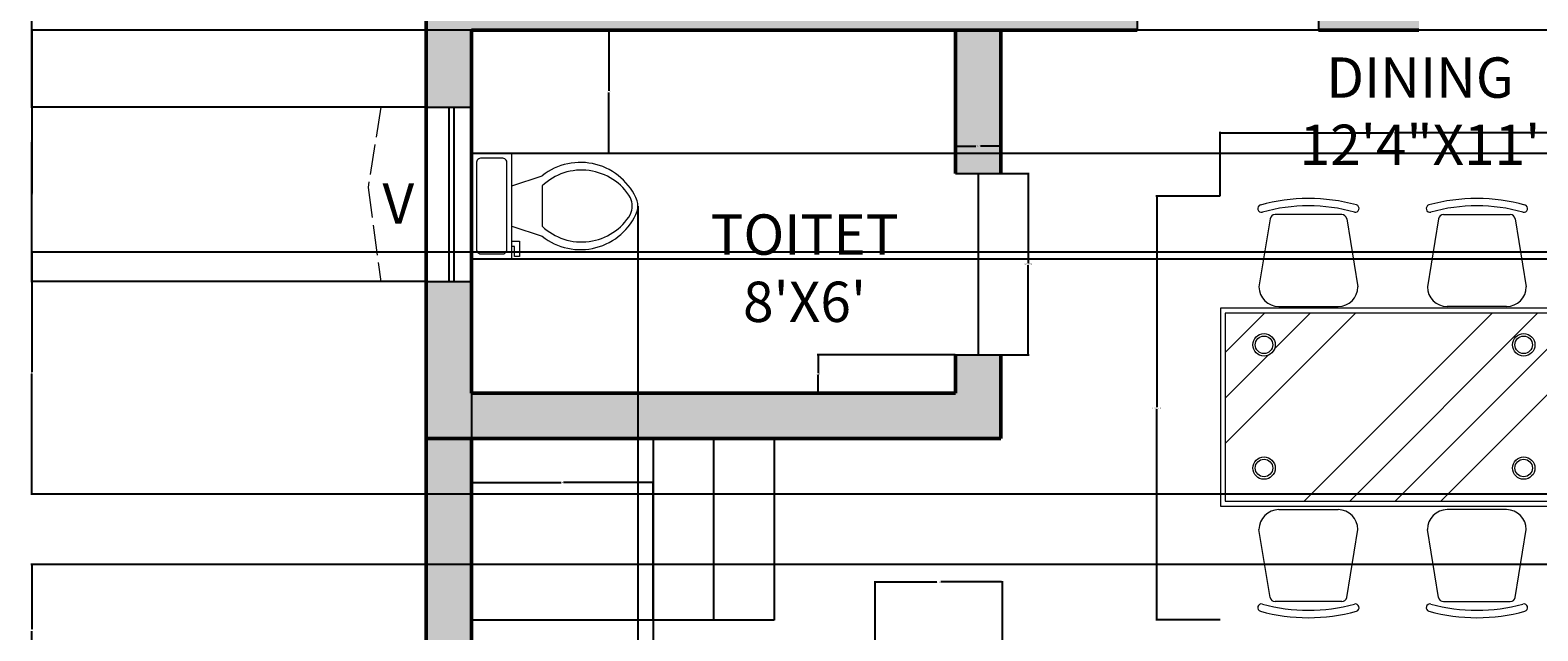
# Model space of a CAD drawing. Units: inches. Extents: x -75 to 416, y -487 to 70.
# Tile 2 of 5: x -75 to 224, y -253 to -133. Entities that reach past the tile are written whole.
import ezdxf

# ---------------------------------------------------------------- set-up
doc = ezdxf.new("R2010")
doc.units = ezdxf.units.IN
doc.header["$MEASUREMENT"] = 0
doc.linetypes.add('ACAD_ISO02W100', pattern=[15, 12, -3])
for name, color, linetype, lineweight in [('A-ANNO-DIMS', 2, 'Continuous', 18), ('A-ANNO-TEXT', 7, 'Continuous', 18), ('A-AREA-IDEN', 7, 'Continuous', 25), ('A-DOOR', 3, 'Continuous', 25), ('A-FLOR-FIXT', 9, 'Continuous', 18), ('A-FLOR-STRS', 7, 'Continuous', 25), ('A-FURN', 8, 'Continuous', 18), ('A-GLAZ', 4, 'Continuous', 25), ('A-GLAZ-OVHD', 4, 'ACAD_ISO02W100', 13), ('A-WALL', 7, 'Continuous', 50), ('A-WALL-PATT', 252, 'Continuous', 13)]:
    doc.layers.add(name, color=color, linetype=linetype, lineweight=lineweight)
doc.styles.get("Standard").update_dxf_attribs({"font": 'arial.ttf'})
doc.dimstyles.get("Standard").update_dxf_attribs({"dimtxt": 0.18, "dimasz": 0.18, "dimexe": 0.18, "dimexo": 0.0625, "dimgap": 0.09, "dimtad": 0, "dimtih": 1, "dimtoh": 1, "dimdec": 4, "dimzin": 0, "dimdsep": 46, "dimtxsty": 'Standard', "dimcen": 0.09, "dimadec": 0, "dimazin": 0, "dimtfac": 1, "dimtdec": 4, "dimtofl": 0, "dimtmove": 0, "dimatfit": 3, "dimfxl": 1, "dimtolj": 1, "dimtzin": 0, "dimarcsym": 0})

# ---------------------------------------------------------------- blocks, each defined once
blk = doc.blocks.new('*U4')
for p, q in [((9.5, -6), (9.5, -2)), ((-10, -8.5), (-8, -8.5)), ((-10, -9.5), (-10, -8.5)), ((-8, -8.5), (-8, -8)), ((-7, -8), (-7, -9.5)), ((-4, -8), (-6, -14)), ((4, -8), (6, -14)), ((-7, -9.5), (-10, -9.5)), ((4, -14), (-4, -14))]:
    blk.add_line(p, q)
blk.add_lwpolyline([(10.5, -8), (10.5, 0), (-10.5, 0), (-10.5, -8)], close=True)
for points in [[(-9.5, -2), (-9.5, -6)], [(8.5, -1), (-8.5, -1)], [(-8.5, -7), (8.5, -7)]]:
    blk.add_lwpolyline(points)
for centre, radius, start, end in [((-8.62, -1.88), 0.884, 81.8699, 188.1301), ((8.62, -1.88), 0.884, 351.8699, 98.1301), ((-8.62, -6.12), 0.884, 171.8699, 278.1301), ((8.62, -6.12), 0.884, 261.8699, 8.1301), ((3.52, -21.58), 12.17, 141.4691, 247.9714), ((4.2, -21.82), 11.33, 136.3677, 238.9468), ((-3.52, -21.58), 12.17, 292.0284, 38.5307), ((-4.2, -21.82), 11.33, 301.053, 43.6321), ((0, -27.88), 4, 245.7318, 294.2682), ((0, -29), 4, 254.8605, 285.1395)]:
    blk.add_arc(centre, radius, start, end)
blk = doc.blocks.new('A$C0FD55737')
for p, q in [((0.2013, 1.6134), (0.1562, 1.3384)), ((0.4912, 1.6302), (0.2211, 1.6302)), ((0.511, 1.6134), (0.5562, 1.3384)), ((0.8828, 1.6134), (0.8376, 1.3384)), ((0.9026, 1.6302), (1.1727, 1.6302)), ((1.1925, 1.6134), (1.2376, 1.3384)), ((0, 1.2513), (0, 0.4513)), ((1.4, 1.2513), (0, 1.2513)), ((0.02, 1.0725), (0.1788, 1.2313)), ((0.02, 0.7043), (0.547, 1.2313)), ((1.38, 1.2313), (0.02, 1.2313)), ((0.02, 1.2313), (0.02, 0.4713)), ((0.2189, 1.0873), (0.3629, 1.2313)), ((0.2362, 1.2584), (0.4762, 1.2584)), ((0.3393, 0.4713), (1.0993, 1.2313)), ((0.5234, 0.4713), (1.2834, 1.2313)), ((1.1576, 1.2584), (0.9176, 1.2584)), ((1.38, 0.4713), (1.38, 1.2313)), ((1.4, 0.4513), (1.4, 1.2513)), ((0.7074, 0.4713), (1.38, 1.1438)), ((0.02, 0.8884), (0.1931, 1.0614)), ((0.8915, 0.4713), (1.38, 0.9597)), ((0, 0.4513), (1.4, 0.4513)), ((0.02, 0.4713), (1.38, 0.4713)), ((0.2362, 0.4371), (0.4762, 0.4371)), ((1.1576, 0.4371), (0.9176, 0.4371)), ((0.2013, 0.0821), (0.1562, 0.3571)), ((0.511, 0.0821), (0.5562, 0.3571)), ((0.8828, 0.0821), (0.8376, 0.3571)), ((1.1925, 0.0821), (1.2376, 0.3571)), ((0.4912, 0.0653), (0.2211, 0.0653)), ((0.9026, 0.0653), (1.1727, 0.0653))]:
    blk.add_line(p, q)
for centre, radius in [((0.1766, 1.1037), 0.0454), ((0.1766, 1.1037), 0.0354), ((1.227, 1.1037), 0.0454), ((1.227, 1.1037), 0.0354), ((0.1766, 0.6052), 0.0454), ((0.1766, 0.6052), 0.0354), ((1.227, 0.6052), 0.0454), ((1.227, 0.6052), 0.0354)]:
    blk.add_circle(centre, radius)
for centre, radius, start, end in [((0.1662, 1.6546), 0.015, 105.49005, 284.28424), ((0.3562, 0.9712), 0.7243, 74.47014, 105.57697), ((0.3562, 0.9716), 0.6939, 74.43245, 105.56755), ((0.5461, 1.6546), 0.015, 255.71576, 74.50995), ((0.8477, 1.6546), 0.015, 105.49005, 284.28424), ((1.0376, 0.9712), 0.7243, 74.42303, 105.52986), ((1.0376, 0.9716), 0.6939, 74.43245, 105.56755), ((1.2276, 1.6546), 0.015, 255.71576, 74.50995), ((0.2211, 1.6102), 0.02, 90, 170.67171), ((0.4912, 1.6102), 0.02, 9.32829, 90), ((0.9026, 1.6102), 0.02, 90, 170.67171), ((1.1727, 1.6102), 0.02, 9.32829, 90), ((0.2362, 1.3384), 0.08, 180, 270), ((0.4762, 1.3384), 0.08, 270, 0), ((0.9176, 1.3384), 0.08, 180, 270), ((1.1576, 1.3384), 0.08, 270, 0), ((0.2362, 0.3571), 0.08, 90, 180), ((0.4762, 0.3571), 0.08, 0, 90), ((0.9176, 0.3571), 0.08, 90, 180), ((1.1576, 0.3571), 0.08, 0, 90), ((0.2211, 0.0853), 0.02, 189.32829, 270), ((0.4912, 0.0853), 0.02, 270, 350.67171), ((0.9026, 0.0853), 0.02, 189.32829, 270), ((1.1727, 0.0853), 0.02, 270, 350.67171), ((0.1662, 0.0409), 0.015, 75.71576, 254.50995), ((0.3562, 0.7243), 0.7243, 254.42303, 285.52986), ((0.3562, 0.7239), 0.6939, 254.43245, 285.56755), ((0.5461, 0.0409), 0.015, 285.49005, 104.28424), ((0.8477, 0.0409), 0.015, 75.71576, 254.50995), ((1.0376, 0.7243), 0.7243, 254.47014, 285.57697), ((1.0376, 0.7239), 0.6939, 254.43245, 285.56755), ((1.2276, 0.0409), 0.015, 285.49005, 104.28424)]:
    blk.add_arc(centre, radius, start, end)
blk = doc.blocks.new('DOOR-36IN')
for p, q in [((0, 9), (0, 0)), ((36, 9), (36, 0)), ((36, 4.5), (0, 4.5))]:
    blk.add_line(p, q)
blk = doc.blocks.new('*D18')
at = {"layer": 'A-ANNO-DIMS', "color": 0, "lineweight": -2, "transparency": 16777216}
for p, q in [((117.62, -161.79), (123.13, -161.79)), ((122.95, -161.97), (122.95, -179.6)), ((122.95, -197.61), (122.95, -179.97)), ((117.62, -197.79), (123.13, -197.79))]:
    blk.add_line(p, q, dxfattribs=at)
at = {"layer": 'A-ANNO-DIMS', "color": 0, "transparency": 16777216}
for points in [[(122.92, -161.97), (122.98, -161.97), (122.95, -161.79)], [(122.92, -197.61), (122.98, -197.61), (122.95, -197.79)]]:
    blk.add_solid(points, dxfattribs=at)
at = {"layer": 'Defpoints', "color": 0, "transparency": 16777216}
for p in [(117.55, -161.79), (122.95, -161.79), (117.55, -197.79)]:
    blk.add_point(p, dxfattribs=at)
at = {"layer": 'A-ANNO-DIMS', "color": 0, "transparency": 16777216, "insert": (122.95, -179.79), "char_height": 0.18, "attachment_point": 5}
blk.add_mtext('\\A1;DOOR 36 TYP.', dxfattribs=at)
blk = doc.blocks.new('*D19')
at = {"layer": 'A-ANNO-DIMS', "color": 0, "lineweight": -2, "transparency": 16777216}
for p, q in [((108.55, -161.72), (108.55, -156.21)), ((108.73, -156.39), (112.59, -156.39)), ((117.37, -156.39), (113.51, -156.39)), ((117.55, -161.72), (117.55, -156.21))]:
    blk.add_line(p, q, dxfattribs=at)
at = {"layer": 'A-ANNO-DIMS', "color": 0, "transparency": 16777216}
for points in [[(108.73, -156.36), (108.73, -156.42), (108.55, -156.39)], [(117.37, -156.36), (117.37, -156.42), (117.55, -156.39)]]:
    blk.add_solid(points, dxfattribs=at)
at = {"layer": 'Defpoints', "color": 0, "transparency": 16777216}
for p in [(108.55, -156.39), (108.55, -161.79), (117.55, -161.79)]:
    blk.add_point(p, dxfattribs=at)
at = {"layer": 'A-ANNO-DIMS', "color": 0, "transparency": 16777216, "insert": (113.05, -156.39), "char_height": 0.18, "attachment_point": 5}
blk.add_mtext('\\A1;9 TYP.', dxfattribs=at)
blk = doc.blocks.new('*D28')
at = {"layer": 'A-ANNO-DIMS', "color": 0, "lineweight": -2, "transparency": 16777216}
for p, q in [((161.02, -166.31), (148.3, -166.31)), ((148.48, -166.49), (148.48, -208.14)), ((148.48, -250.15), (148.48, -208.51)), ((161.02, -250.33), (148.3, -250.33))]:
    blk.add_line(p, q, dxfattribs=at)
at = {"layer": 'A-ANNO-DIMS', "color": 0, "transparency": 16777216}
for points in [[(148.45, -166.49), (148.51, -166.49), (148.48, -166.31)], [(148.45, -250.15), (148.51, -250.15), (148.48, -250.33)]]:
    blk.add_solid(points, dxfattribs=at)
at = {"layer": 'Defpoints', "color": 0, "transparency": 16777216}
for p in [(148.48, -166.31), (161.08, -166.31), (161.08, -250.33)]:
    blk.add_point(p, dxfattribs=at)
at = {"layer": 'A-ANNO-DIMS', "color": 0, "transparency": 16777216, "insert": (148.48, -208.32), "char_height": 0.18, "attachment_point": 5}
blk.add_mtext('\\A1;DINING SET 84', dxfattribs=at)
blk = doc.blocks.new('*D29')
at = {"layer": 'A-ANNO-DIMS', "color": 0, "lineweight": -2, "transparency": 16777216}
for p, q in [((161.08, -166.25), (161.08, -153.53)), ((161.26, -153.71), (195.2, -153.71)), ((229.56, -153.71), (195.63, -153.71)), ((229.74, -166.25), (229.74, -153.53))]:
    blk.add_line(p, q, dxfattribs=at)
at = {"layer": 'A-ANNO-DIMS', "color": 0, "transparency": 16777216}
for points in [[(161.26, -153.68), (161.26, -153.74), (161.08, -153.71)], [(229.56, -153.68), (229.56, -153.74), (229.74, -153.71)]]:
    blk.add_solid(points, dxfattribs=at)
at = {"layer": 'Defpoints', "color": 0, "transparency": 16777216}
for p in [(229.74, -153.71), (161.08, -166.31), (229.74, -166.31)]:
    blk.add_point(p, dxfattribs=at)
at = {"layer": 'A-ANNO-DIMS', "color": 0, "transparency": 16777216, "insert": (195.41, -153.71), "char_height": 0.18, "attachment_point": 5}
blk.add_mtext('\\A1;69', dxfattribs=at)
blk = doc.blocks.new('*D44')
at = {"layer": 'A-ANNO-DIMS', "color": 0, "lineweight": -2, "transparency": 16777216}
for p, q in [((3.49, -71.81), (-74.89, -71.81)), ((-74.71, -71.99), (-74.71, -110.05)), ((-74.71, -148.46), (-74.71, -110.41)), ((3.49, -148.64), (-74.89, -148.64))]:
    blk.add_line(p, q, dxfattribs=at)
at = {"layer": 'A-ANNO-DIMS', "color": 0, "transparency": 16777216}
for points in [[(-74.74, -71.99), (-74.68, -71.99), (-74.71, -71.81)], [(-74.74, -148.46), (-74.68, -148.46), (-74.71, -148.64)]]:
    blk.add_solid(points, dxfattribs=at)
at = {"layer": 'Defpoints', "color": 0, "transparency": 16777216}
for p in [(3.55, -71.81), (-74.71, -148.64), (3.55, -148.64)]:
    blk.add_point(p, dxfattribs=at)
at = {"layer": 'A-ANNO-DIMS', "color": 0, "transparency": 16777216, "insert": (-74.71, -110.23), "char_height": 0.18, "attachment_point": 5}
blk.add_mtext('\\A1;76.83', dxfattribs=at)
blk = doc.blocks.new('*D45')
at = {"layer": 'A-ANNO-DIMS', "color": 0, "lineweight": -2, "transparency": 16777216}
for p, q in [((3.49, -148.64), (-74.89, -148.64)), ((-74.71, -148.82), (-74.71, -165.75)), ((-74.71, -183.05), (-74.71, -166.12)), ((3.49, -183.23), (-74.89, -183.23))]:
    blk.add_line(p, q, dxfattribs=at)
at = {"layer": 'A-ANNO-DIMS', "color": 0, "transparency": 16777216}
for points in [[(-74.74, -148.82), (-74.68, -148.82), (-74.71, -148.64)], [(-74.74, -183.05), (-74.68, -183.05), (-74.71, -183.23)]]:
    blk.add_solid(points, dxfattribs=at)
at = {"layer": 'Defpoints', "color": 0, "transparency": 16777216}
for p in [(3.55, -148.64), (-74.71, -183.23), (3.55, -183.23)]:
    blk.add_point(p, dxfattribs=at)
at = {"layer": 'A-ANNO-DIMS', "color": 0, "transparency": 16777216, "insert": (-74.71, -165.94), "char_height": 0.18, "attachment_point": 5}
blk.add_mtext('\\A1;34.59', dxfattribs=at)
blk = doc.blocks.new('*D52')
at = {"layer": 'A-ANNO-DIMS', "color": 0, "lineweight": -2, "transparency": 16777216}
for p, q in [((260.49, -133.37), (-74.89, -133.37)), ((-74.71, -133.55), (-74.71, -155.19)), ((-74.71, -177.19), (-74.71, -155.55)), ((260.49, -177.37), (-74.89, -177.37))]:
    blk.add_line(p, q, dxfattribs=at)
at = {"layer": 'A-ANNO-DIMS', "color": 0, "transparency": 16777216}
for points in [[(-74.74, -133.55), (-74.68, -133.55), (-74.71, -133.37)], [(-74.74, -177.19), (-74.68, -177.19), (-74.71, -177.37)]]:
    blk.add_solid(points, dxfattribs=at)
at = {"layer": 'Defpoints', "color": 0, "transparency": 16777216}
for p in [(260.55, -133.37), (-74.71, -177.37), (260.55, -177.37)]:
    blk.add_point(p, dxfattribs=at)
at = {"layer": 'A-ANNO-DIMS', "color": 0, "transparency": 16777216, "insert": (-74.71, -155.37), "char_height": 0.18, "attachment_point": 5}
blk.add_mtext('\\A1;43.99', dxfattribs=at)
blk = doc.blocks.new('*D53')
at = {"layer": 'A-ANNO-DIMS', "color": 0, "lineweight": -2, "transparency": 16777216}
for p, q in [((260.49, -177.37), (-74.89, -177.37)), ((-74.71, -177.55), (-74.71, -201.19)), ((-74.71, -225.19), (-74.71, -201.55)), ((260.49, -225.37), (-74.89, -225.37))]:
    blk.add_line(p, q, dxfattribs=at)
at = {"layer": 'A-ANNO-DIMS', "color": 0, "transparency": 16777216}
for points in [[(-74.74, -177.55), (-74.68, -177.55), (-74.71, -177.37)], [(-74.74, -225.19), (-74.68, -225.19), (-74.71, -225.37)]]:
    blk.add_solid(points, dxfattribs=at)
at = {"layer": 'Defpoints', "color": 0, "transparency": 16777216}
for p in [(260.55, -177.37), (-74.71, -225.37), (260.55, -225.37)]:
    blk.add_point(p, dxfattribs=at)
at = {"layer": 'A-ANNO-DIMS', "color": 0, "transparency": 16777216, "insert": (-74.71, -201.37), "char_height": 0.18, "attachment_point": 5}
blk.add_mtext('\\A1;48', dxfattribs=at)
blk = doc.blocks.new('*D55')
at = {"layer": 'A-ANNO-DIMS', "color": 0, "lineweight": -2, "transparency": 16777216}
for p, q in [((269.49, -239.36), (-74.89, -239.36)), ((-74.71, -239.54), (-74.71, -252.19)), ((-74.71, -265.19), (-74.71, -252.55)), ((269.49, -265.37), (-74.89, -265.37))]:
    blk.add_line(p, q, dxfattribs=at)
at = {"layer": 'A-ANNO-DIMS', "color": 0, "transparency": 16777216}
for points in [[(-74.74, -239.54), (-74.68, -239.54), (-74.71, -239.36)], [(-74.74, -265.19), (-74.68, -265.19), (-74.71, -265.37)]]:
    blk.add_solid(points, dxfattribs=at)
at = {"layer": 'Defpoints', "color": 0, "transparency": 16777216}
for p in [(269.55, -239.36), (-74.71, -265.37), (269.55, -265.37)]:
    blk.add_point(p, dxfattribs=at)
at = {"layer": 'A-ANNO-DIMS', "color": 0, "transparency": 16777216, "insert": (-74.71, -252.37), "char_height": 0.18, "attachment_point": 5}
blk.add_mtext('\\A1;26.01', dxfattribs=at)
blk = doc.blocks.new('*D58')
at = {"layer": 'A-ANNO-DIMS', "color": 0, "lineweight": -2, "transparency": 16777216}
for p, q in [((108.49, -197.79), (81.11, -197.79)), ((81.29, -197.97), (81.29, -201.4)), ((81.29, -205.19), (81.29, -201.76)), ((108.49, -205.37), (81.11, -205.37))]:
    blk.add_line(p, q, dxfattribs=at)
at = {"layer": 'A-ANNO-DIMS', "color": 0, "transparency": 16777216}
for points in [[(81.26, -197.97), (81.32, -197.97), (81.29, -197.79)], [(81.26, -205.19), (81.32, -205.19), (81.29, -205.37)]]:
    blk.add_solid(points, dxfattribs=at)
at = {"layer": 'Defpoints', "color": 0, "transparency": 16777216}
for p in [(81.29, -197.79), (108.55, -197.79), (108.55, -205.37)]:
    blk.add_point(p, dxfattribs=at)
at = {"layer": 'A-ANNO-DIMS', "color": 0, "transparency": 16777216, "insert": (81.29, -201.58), "char_height": 0.18, "attachment_point": 5}
blk.add_mtext('\\A1;7.588', dxfattribs=at)
blk = doc.blocks.new('*D60')
at = {"layer": 'A-ANNO-DIMS', "color": 0, "lineweight": -2, "transparency": 16777216}
for p, q in [((12.62, -157.75), (415.9, -157.75)), ((415.72, -157.93), (415.72, -168.07)), ((415.72, -178.57), (415.72, -168.43)), ((12.62, -178.75), (415.9, -178.75))]:
    blk.add_line(p, q, dxfattribs=at)
at = {"layer": 'A-ANNO-DIMS', "color": 0, "transparency": 16777216}
for points in [[(415.69, -157.93), (415.75, -157.93), (415.72, -157.75)], [(415.69, -178.57), (415.75, -178.57), (415.72, -178.75)]]:
    blk.add_solid(points, dxfattribs=at)
at = {"layer": 'Defpoints', "color": 0, "transparency": 16777216}
for p in [(12.55, -157.75), (12.55, -178.75), (415.72, -178.75)]:
    blk.add_point(p, dxfattribs=at)
at = {"layer": 'A-ANNO-DIMS', "color": 0, "transparency": 16777216, "insert": (415.72, -168.25), "char_height": 0.18, "attachment_point": 5}
blk.add_mtext('\\A1;21', dxfattribs=at)
blk = doc.blocks.new('*D61')
at = {"layer": 'A-ANNO-DIMS', "color": 0, "lineweight": -2, "transparency": 16777216}
for p, q in [((12.62, -133.37), (39.99, -133.37)), ((39.81, -133.55), (39.81, -145.38)), ((39.81, -157.57), (39.81, -145.75)), ((12.62, -157.75), (39.99, -157.75))]:
    blk.add_line(p, q, dxfattribs=at)
at = {"layer": 'A-ANNO-DIMS', "color": 0, "transparency": 16777216}
for points in [[(39.78, -133.55), (39.84, -133.55), (39.81, -133.37)], [(39.78, -157.57), (39.84, -157.57), (39.81, -157.75)]]:
    blk.add_solid(points, dxfattribs=at)
at = {"layer": 'Defpoints', "color": 0, "transparency": 16777216}
for p in [(12.55, -133.37), (12.55, -157.75), (39.81, -157.75)]:
    blk.add_point(p, dxfattribs=at)
at = {"layer": 'A-ANNO-DIMS', "color": 0, "transparency": 16777216, "insert": (39.81, -145.56), "char_height": 0.18, "attachment_point": 5}
blk.add_mtext('\\A1;24.38', dxfattribs=at)
blk = doc.blocks.new('*D62')
at = {"layer": 'A-ANNO-DIMS', "color": 0, "lineweight": -2, "transparency": 16777216}
for p, q in [((12.55, -250.31), (12.55, -222.93)), ((12.73, -223.11), (30.33, -223.11)), ((48.37, -223.11), (30.77, -223.11)), ((48.55, -250.31), (48.55, -222.93))]:
    blk.add_line(p, q, dxfattribs=at)
at = {"layer": 'A-ANNO-DIMS', "color": 0, "transparency": 16777216}
for points in [[(12.73, -223.08), (12.73, -223.14), (12.55, -223.11)], [(48.37, -223.08), (48.37, -223.14), (48.55, -223.11)]]:
    blk.add_solid(points, dxfattribs=at)
at = {"layer": 'Defpoints', "color": 0, "transparency": 16777216}
for p in [(48.55, -223.11), (12.55, -250.37), (48.55, -250.37)]:
    blk.add_point(p, dxfattribs=at)
at = {"layer": 'A-ANNO-DIMS', "color": 0, "transparency": 16777216, "insert": (30.55, -223.11), "char_height": 0.18, "attachment_point": 5}
blk.add_mtext('\\A1;36', dxfattribs=at)
blk = doc.blocks.new('*D64')
at = {"layer": 'A-ANNO-DIMS', "color": 0, "lineweight": -2, "transparency": 16777216}
for p, q in [((92.6, -270.01), (92.6, -242.63)), ((92.78, -242.81), (104.83, -242.81)), ((117.66, -242.81), (105.62, -242.81)), ((117.84, -270.01), (117.84, -242.63))]:
    blk.add_line(p, q, dxfattribs=at)
at = {"layer": 'A-ANNO-DIMS', "color": 0, "transparency": 16777216}
for points in [[(92.78, -242.78), (92.78, -242.84), (92.6, -242.81)], [(117.66, -242.78), (117.66, -242.84), (117.84, -242.81)]]:
    blk.add_solid(points, dxfattribs=at)
at = {"layer": 'Defpoints', "color": 0, "transparency": 16777216}
for p in [(117.84, -242.81), (92.6, -270.07), (117.84, -270.07)]:
    blk.add_point(p, dxfattribs=at)
at = {"layer": 'A-ANNO-DIMS', "color": 0, "transparency": 16777216, "insert": (105.22, -242.81), "char_height": 0.18, "attachment_point": 5}
blk.add_mtext('\\A1;25.24', dxfattribs=at)
blk = doc.blocks.new('*D70')
at = {"layer": 'A-ANNO-DIMS', "color": 0, "lineweight": -2, "transparency": 16777216}
for p, q in [((45.55, -168.31), (45.55, -486.72)), ((12.55, -178.81), (12.55, -486.72)), ((12.73, -486.54), (28.83, -486.54)), ((45.37, -486.54), (29.27, -486.54))]:
    blk.add_line(p, q, dxfattribs=at)
at = {"layer": 'A-ANNO-DIMS', "color": 0, "transparency": 16777216}
for points in [[(12.73, -486.51), (12.73, -486.57), (12.55, -486.54)], [(45.37, -486.51), (45.37, -486.57), (45.55, -486.54)]]:
    blk.add_solid(points, dxfattribs=at)
at = {"layer": 'Defpoints', "color": 0, "transparency": 16777216}
for p in [(45.55, -168.25), (12.55, -178.75), (45.55, -486.54)]:
    blk.add_point(p, dxfattribs=at)
at = {"layer": 'A-ANNO-DIMS', "color": 0, "transparency": 16777216, "insert": (29.05, -486.54), "char_height": 0.18, "attachment_point": 5}
blk.add_mtext('\\A1;33', dxfattribs=at)

msp = doc.modelspace()

# ---------------------------------------------------------------- hatches: boundary and pattern name
at = {"layer": 'A-WALL-PATT'}
h = msp.add_hatch(color=256, dxfattribs=at)
h.dxf.hatch_style = 1
h.paths.add_polyline_path([(84.8603, 28.6255), (3.5531, 28.6255), (3.5531, -23.8141), (12.5531, -23.8141), (12.5531, 19.6255), (84.8603, 19.6255)])
h.paths.add_polyline_path([(263.7442, 28.6255), (132.8603, 28.6255), (132.8603, 19.6255), (146.5531, 19.6255), (180.5531, 19.6255), (180.5531, -124.3745), (180.5531, -133.3745), (200.467, -133.3745), (200.467, -124.3745), (189.5531, -124.3745), (189.5531, 19.6255), (263.7442, 19.6255)])
h.paths.add_polyline_path([(374.5531, 28.6255), (311.7442, 28.6255), (311.7442, 19.6255), (327.5531, 19.6255), (365.5531, 19.6255), (365.5531, -37.0191), (374.5531, -37.0191)])
h.paths.add_polyline_path([(144.5531, -124.3745), (12.5531, -124.3745), (12.5531, -71.8141), (3.5531, -71.8141), (3.5531, -148.6403), (12.5531, -148.6403), (12.5531, -133.3745), (144.5531, -133.3745)])
h.paths.add_polyline_path([(117.5531, -133.3745), (108.5531, -133.3745), (108.5531, -161.7866), (117.5531, -161.7866)])
h.paths.add_polyline_path([(374.5531, -85.0191), (365.5531, -85.0191), (365.5531, -124.3745), (236.467, -124.3745), (236.467, -133.3745), (374.5531, -133.3745)])
h.paths.add_polyline_path([(374.5531, -133.3745), (365.5531, -133.3745), (365.5531, -183.1692), (374.5531, -183.1692)])
h.paths.add_polyline_path([(374.5531, -231.1692), (365.5531, -231.1692), (365.5531, -265.3745), (260.5531, -265.3745), (260.5531, -274.3745), (374.5531, -274.3745)])
h.paths.add_polyline_path([(260.5531, -265.3745), (215.5531, -265.3745), (215.5531, -288.4908), (224.5531, -288.4908), (224.5531, -274.3745), (260.5531, -274.3745)])
h.paths.add_polyline_path([(374.5531, -274.3745), (365.5531, -274.3745), (365.5531, -345.9302), (374.5531, -345.9302)])
h.paths.add_polyline_path([(374.5531, -393.9302), (365.5531, -393.9302), (365.5531, -436.3745), (321.1982, -436.3745), (321.1982, -445.3745), (374.5531, -445.3745)])
h.paths.add_polyline_path([(224.5531, -324.4908), (215.5531, -324.4908), (215.5531, -445.3745), (273.1982, -445.3745), (273.1982, -436.3745), (265.0531, -436.3745), (245.0531, -436.3745), (224.5531, -436.3745)])
h.paths.add_polyline_path([(12.5531, -183.233), (3.5531, -183.233), (3.5531, -214.3745), (117.5531, -214.3745), (117.5531, -197.7866), (108.5531, -197.7866), (108.5531, -205.3745), (12.5531, -205.3745)])
h.paths.add_polyline_path([(12.5531, -214.3745), (3.5531, -214.3745), (3.5531, -290.2477), (12.5531, -290.2477)])
h.paths.add_polyline_path([(75.0426, -381.3745), (12.5531, -381.3745), (12.5531, -350.2477), (3.5531, -350.2477), (3.5531, -390.3745), (75.0426, -390.3745)])
h.paths.add_polyline_path([(154.4537, -381.3745), (123.0426, -381.3745), (123.0426, -390.3745), (154.4537, -390.3745)])
h.paths.add_polyline_path([(215.5531, -381.3745), (202.4537, -381.3745), (202.4537, -390.3745), (215.5531, -390.3745)])

# ---------------------------------------------------------------- linework, layer by layer
at = {"layer": 'A-FLOR-STRS'}
for p, q in [((48.5531, -214.3745), (48.5531, -250.3745)), ((60.5531, -214.3745), (60.5531, -250.3745)), ((72.5531, -214.3745), (72.5531, -250.3745)), ((48.5531, -250.3745), (12.5531, -250.3745)), ((72.5531, -250.3745), (48.5531, -250.3745)), ((48.5531, -250.3745), (48.5531, -345.3745))]:
    msp.add_line(p, q, dxfattribs=at)
at = {"layer": 'A-GLAZ'}
for p, q in [((3.5531, -148.6403), (12.5531, -148.6403)), ((8.0531, -148.6403), (8.0531, -183.233)), ((9.0531, -148.6403), (9.0531, -183.233)), ((3.5531, -183.233), (12.5531, -183.233))]:
    msp.add_line(p, q, dxfattribs=at)
at = {"layer": 'A-GLAZ-OVHD', "ltscale": 0.5}
for p, q in [((-5.4469, -148.6403), (-7.9877, -164.6033)), ((3.5531, -148.6403), (-5.4469, -148.6403)), ((-7.9877, -164.6033), (-5.4469, -183.233)), ((-5.4469, -183.233), (3.5531, -183.233))]:
    msp.add_line(p, q, dxfattribs=at)
at = {"layer": 'A-WALL'}
for p, q in [((3.5531, 28.6255), (3.5531, -390.3745)), ((12.5531, -133.3745), (144.5531, -133.3745)), ((12.5531, -133.3745), (12.5531, -205.3745)), ((108.5531, -133.3745), (108.5531, -161.7866)), ((117.5531, -133.3745), (117.5531, -161.7866)), ((180.5531, -133.3745), (200.467, -133.3745)), ((108.5531, -197.7866), (108.5531, -205.3745)), ((117.5531, -197.7866), (117.5531, -214.3745)), ((12.5531, -205.3745), (108.5531, -205.3745)), ((3.5531, -214.3745), (117.5531, -214.3745)), ((12.5531, -214.3745), (12.5531, -381.3745))]:
    msp.add_line(p, q, dxfattribs=at)

# ---------------------------------------------------------------- block references
at = {"layer": 'A-DOOR'}
msp.add_blockref('DOOR-36IN', (144.553, -133.374), dxfattribs=at)
at = {"layer": 'A-DOOR', "rotation": 89.99999999999996}
msp.add_blockref('DOOR-36IN', (117.5526, -197.7867), dxfattribs=at)
at = {"layer": 'A-FLOR-FIXT', "rotation": 90}
msp.add_blockref('*U4', (12.5531, -168.2524), dxfattribs=at)
at = {"layer": 'A-FURN', "xscale": 49.04285923157839, "yscale": 49.04285923157839, "zscale": 49.04285923157839}
msp.add_blockref('A$C0FD55737', (161.0849, -249.899), dxfattribs=at)

# ---------------------------------------------------------------- texts
at = {"layer": 'A-ANNO-TEXT', "insert": (-9.5498, -163.7476), "char_height": 8, "attachment_point": 1}
msp.add_mtext_dynamic_manual_height_columns('\\pxqc;V', width=15.130285, gutter_width=1, heights=[0], dxfattribs=at)
at = {"layer": 'A-AREA-IDEN', "char_height": 8, "attachment_point": 1}
for s, insert in [('\\pxqc;DINING\\P12\'4"X11\'', (128.5101, -138.7785)), ("\\pxqc;TOITET\\P8'X6'", (6.4335, -169.9113))]:
    msp.add_mtext_dynamic_manual_height_columns(s, width=144.357858, gutter_width=1, heights=[0], dxfattribs=dict(at, insert=insert))

# ---------------------------------------------------------------- dimensions: what is measured, and where the dimension line sits
at = {"layer": 'A-ANNO-DIMS'}
for base, p1, p2, angle, override, picture, middle in [((-74.7069, -148.6403), (3.5531, -71.8141), (3.5531, -148.6403), 90, {"dimdec": 2, "dimlfac": 1, "dimrnd": 0, "dimzin": 0, "dimdsep": 46, "dimlunit": 2}, '*D44', (-74.7069, -110.2272)), ((-74.7069, -177.367), (260.5531, -133.3745), (260.5531, -177.367), 90, {"dimdec": 2, "dimlfac": 1, "dimrnd": 0, "dimzin": 0, "dimdsep": 46, "dimlunit": 2}, '*D52', (-74.7069, -155.3707)), ((39.8131, -157.7524), (12.5531, -133.3745), (12.5531, -157.7524), 270, {"dimdec": 2, "dimlfac": 1, "dimrnd": 0, "dimzin": 0, "dimdsep": 46, "dimlunit": 2}, '*D61', (39.8131, -145.5635)), ((-74.7069, -183.233), (3.5531, -148.6403), (3.5531, -183.233), 90, {"dimdec": 2, "dimlfac": 1, "dimrnd": 0, "dimzin": 0, "dimdsep": 46, "dimlunit": 2}, '*D45', (-74.7069, -165.9367)), ((415.7227, -178.7524), (12.5531, -157.7524), (12.5531, -178.7524), 90, {"dimdec": 0, "dimlfac": 1, "dimrnd": 0, "dimzin": 0, "dimdsep": 46, "dimlunit": 2}, '*D60', (415.7227, -168.2524)), ((-74.7069, -225.367), (260.5531, -177.367), (260.5531, -225.367), 90, {"dimdec": 0, "dimlfac": 1, "dimrnd": 0, "dimzin": 0, "dimdsep": 46, "dimlunit": 2}, '*D53', (-74.7069, -201.367)), ((81.2931, -197.7866), (108.5531, -205.3745), (108.5531, -197.7866), 90, {"dimdec": 3, "dimlfac": 1, "dimrnd": 0, "dimzin": 0, "dimdsep": 46, "dimlunit": 2}, '*D58', (81.2931, -201.5806)), ((-74.7069, -265.3745), (269.5531, -239.362), (269.5531, -265.3745), 90, {"dimdec": 2, "dimlfac": 1, "dimrnd": 0, "dimzin": 0, "dimdsep": 46, "dimlunit": 2}, '*D55', (-74.7069, -252.3682))]:
    dim = msp.add_linear_dim(base=base, p1=p1, p2=p2, angle=angle, dimstyle='Standard', override=override, dxfattribs=at)
    dim.commit()
    dim.dimension.update_dxf_attribs({"geometry": picture, "text_midpoint": middle})
for base, p1, p2, override, picture, middle in [((229.745, -153.7078), (161.085, -166.3112), (229.745, -166.3112), {"dimdec": 0, "dimlfac": 1, "dimrnd": 0, "dimzin": 0, "dimdsep": 46, "dimlunit": 2}, '*D29', (195.415, -153.7078)), ((45.553, -486.5442), (12.5531, -178.7524), (45.553, -168.2524), {"dimdec": 0, "dimlfac": 1, "dimrnd": 0, "dimzin": 0, "dimdsep": 46, "dimlunit": 2}, '*D70', (29.053, -486.5442)), ((48.5531, -223.1145), (12.5531, -250.3745), (48.5531, -250.3745), {"dimdec": 0, "dimlfac": 1, "dimrnd": 0, "dimzin": 0, "dimdsep": 46, "dimlunit": 2}, '*D62', (30.5531, -223.1145)), ((117.8408, -242.8127), (92.6027, -270.0727), (117.8408, -270.0727), {"dimdec": 2, "dimlfac": 1, "dimrnd": 0, "dimzin": 0, "dimdsep": 46, "dimlunit": 2}, '*D64', (105.2218, -242.8127))]:
    dim = msp.add_linear_dim(base=base, p1=p1, p2=p2, dimstyle='Standard', override=override, dxfattribs=at)
    dim.commit()
    dim.dimension.update_dxf_attribs({"geometry": picture, "text_midpoint": middle})
for base, p1, p2, angle, text, picture, middle in [((108.5531, -156.3866), (117.5531, -161.7866), (108.5531, -161.7866), 180, '<> TYP.', '*D19', (113.0531, -156.3866)), ((122.9531, -161.7866), (117.5531, -197.7866), (117.5531, -161.7866), 90, 'DOOR <> TYP.', '*D18', (122.9531, -179.7866)), ((148.4815, -166.3112), (161.085, -250.3339), (161.085, -166.3112), 90, 'DINING SET <>', '*D28', (148.4815, -208.3225))]:
    dim = msp.add_linear_dim(base=base, p1=p1, p2=p2, angle=angle, text=text, dimstyle='Standard', override={"dimdec": 0, "dimlfac": 1, "dimrnd": 0, "dimzin": 0, "dimdsep": 46, "dimlunit": 2}, dxfattribs=at)
    dim.commit()
    dim.dimension.update_dxf_attribs({"geometry": picture, "text_midpoint": middle})

doc.saveas('drawing.dxf')
